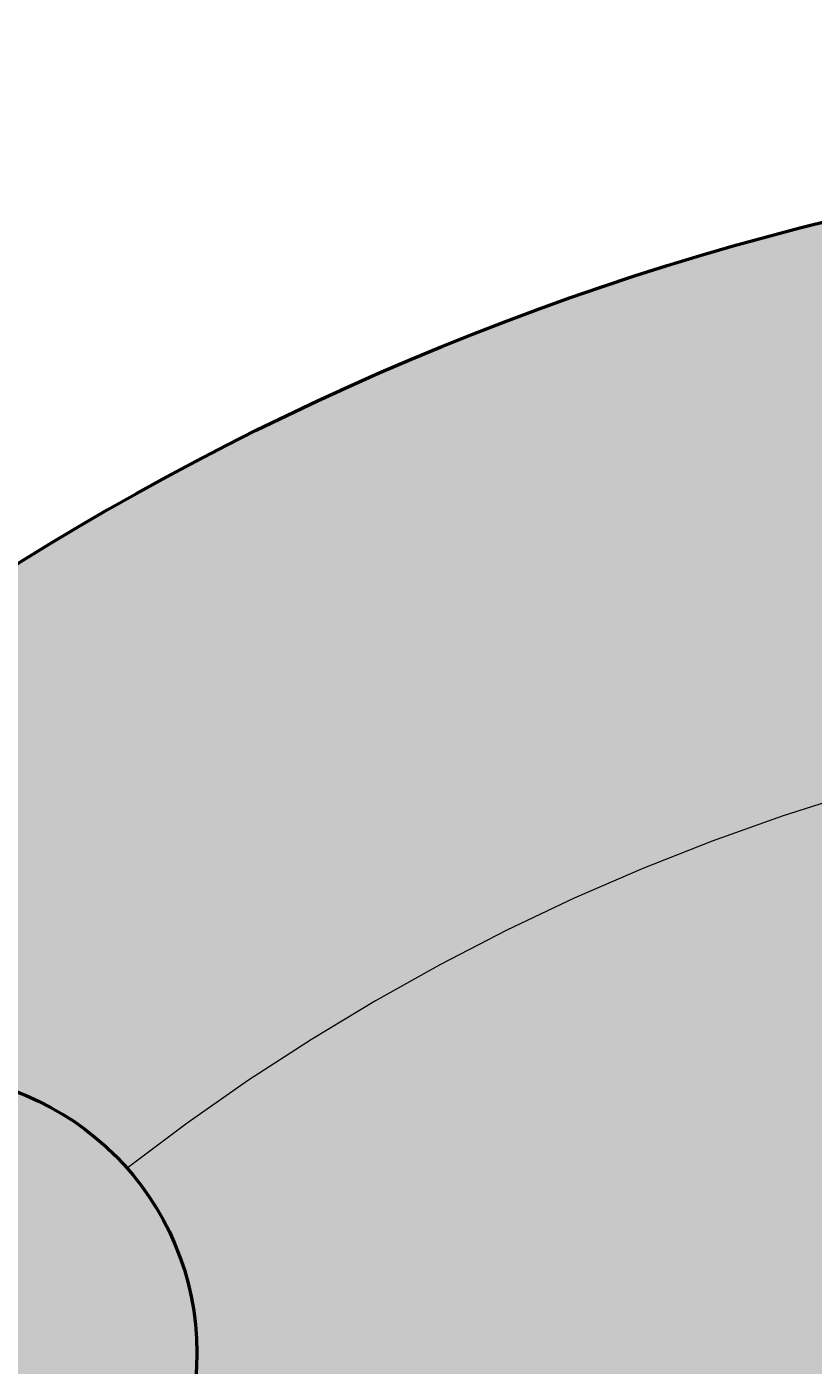
# Model space of a CAD drawing. Units: inches. Extents: x 139261 to 139415, y 52839 to 52963.
# Tile 17 of 20: x 139314 to 139328, y 52928 to 52952. Entities that reach past the tile are written whole.
import ezdxf

# ---------------------------------------------------------------- set-up
doc = ezdxf.new("R2010")
doc.units = ezdxf.units.IN
doc.header["$MEASUREMENT"] = 0
doc.linetypes.add('CENTER', pattern=[50.8, 31.75, -6.35, 6.35, -6.35])
for name, color, linetype, lineweight in [('M-CNTR', 4, 'CENTER', 18), ('M-DIMS', 2, 'Continuous', 25), ('M-HATC', 8, 'Continuous', 18), ('M-OUTL', 7, 'Continuous', 50)]:
    doc.layers.add(name, color=color, linetype=linetype, lineweight=lineweight)
doc.styles.get("Standard").update_dxf_attribs({"font": 'arial.ttf'})
doc.dimstyles.get("Standard").update_dxf_attribs({"dimtxt": 0.18, "dimasz": 0.18, "dimexe": 0.18, "dimexo": 0.0625, "dimgap": 0.09, "dimtad": 0, "dimtih": 1, "dimtoh": 1, "dimdec": 4, "dimzin": 0, "dimdsep": 46, "dimtxsty": 'Standard', "dimcen": 0.09, "dimadec": 0, "dimazin": 0, "dimtfac": 1, "dimtdec": 4, "dimtofl": 0, "dimtmove": 0, "dimatfit": 3, "dimfxl": 1, "dimtolj": 1, "dimtzin": 0, "dimarcsym": 0})

# ---------------------------------------------------------------- blocks, each defined once
blk = doc.blocks.new('*U1')
blk.add_circle((0, 0), 5)
blk = doc.blocks.new('*U2')
at = {"layer": 'M-OUTL', "color": 0, "linetype": 'ByBlock', "lineweight": -2, "transparency": 16777216, "rotation": 45.00000000000001}
blk.add_blockref('*U1', (139312.073, 52928.502), dxfattribs=at)
blk = doc.blocks.new('*D4')
at = {"layer": 'Defpoints', "color": 0, "transparency": 16777216}
for p in [(139373.053, 52923.26), (139307.661, 52877.175)]:
    blk.add_point(p, dxfattribs=at)
at = {"layer": 'M-DIMS', "color": 0, "lineweight": -2, "transparency": 16777216}
for p, q in [((139414.011, 52952.126), (139373.2, 52923.364)), ((139414.191, 52952.126), (139414.011, 52952.126)), ((139340.267, 52900.217), (139340.447, 52900.217)), ((139340.357, 52900.127), (139340.357, 52900.307))]:
    blk.add_line(p, q, dxfattribs=at)
blk.add_arc((139340.357, 52900.217), 40, 34.9168, 52.0771, dxfattribs=at)
at = {"layer": 'M-DIMS', "color": 0, "transparency": 16777216}
blk.add_solid([(139373.183, 52923.388), (139373.217, 52923.339), (139373.053, 52923.26)], dxfattribs=at)
at = {"layer": 'M-DIMS', "color": 0, "transparency": 16777216, "insert": (139414.822, 52952.126), "char_height": 0.18, "attachment_point": 5}
blk.add_mtext('\\A1;∅80.0000', dxfattribs=at)
blk = doc.blocks.new('*D9')
at = {"layer": 'Defpoints', "color": 0, "transparency": 16777216}
for p in [(139302.054, 52932.357), (139378.659, 52868.078)]:
    blk.add_point(p, dxfattribs=at)
at = {"layer": 'M-DIMS', "color": 0, "lineweight": -2, "transparency": 16777216}
for p, q in [((139278.893, 52951.64), (139279.073, 52951.64)), ((139279.073, 52951.64), (139301.916, 52932.472)), ((139340.267, 52900.217), (139340.447, 52900.217)), ((139340.357, 52900.127), (139340.357, 52900.307))]:
    blk.add_line(p, q, dxfattribs=at)
at = {"layer": 'M-DIMS', "color": 0, "transparency": 16777216}
blk.add_solid([(139301.936, 52932.495), (139301.897, 52932.449), (139302.054, 52932.357)], dxfattribs=at)
at = {"layer": 'M-DIMS', "color": 0, "transparency": 16777216, "insert": (139278.506, 52951.64), "char_height": 0.18, "attachment_point": 5}
blk.add_mtext('\\A1;∅100', dxfattribs=at)
blk = doc.blocks.new('*D10')
at = {"layer": 'Defpoints', "color": 0, "transparency": 16777216}
for p in [(139325.07, 52937.181), (139355.644, 52863.254)]:
    blk.add_point(p, dxfattribs=at)
at = {"layer": 'M-DIMS', "color": 0, "lineweight": -2, "transparency": 16777216}
for p, q in [((139340.267, 52900.217), (139340.447, 52900.217)), ((139340.357, 52900.127), (139340.357, 52900.307)), ((139364.816, 52841.075), (139355.712, 52863.087)), ((139364.996, 52841.075), (139364.816, 52841.075))]:
    blk.add_line(p, q, dxfattribs=at)
at = {"layer": 'M-DIMS', "color": 0, "transparency": 16777216}
blk.add_solid([(139355.74, 52863.099), (139355.685, 52863.076), (139355.644, 52863.254)], dxfattribs=at)
at = {"layer": 'M-DIMS', "color": 0, "transparency": 16777216, "insert": (139365.312, 52841.075), "char_height": 0.18, "attachment_point": 5}
blk.add_mtext('\\A1;∅80', dxfattribs=at)

msp = doc.modelspace()

# ---------------------------------------------------------------- hatches: boundary and pattern name
at = {"layer": 'M-HATC'}
h = msp.add_hatch(color=256, dxfattribs=at)
h.dxf.hatch_style = 1
h.paths.add_polyline_path([(139290.35689, 52900.21749, 1), (139390.35689, 52900.21749, 1)])
h.paths.add_polyline_path([(139335.36666, 52939.90499, -0.01563646), (139335.35689, 52940.21749, -1), (139345.35689, 52940.21749, -0.01563646), (139345.34711, 52939.90499, -0.13461315), (139364.89157, 52931.80941, -0.691035), (139373.64116, 52928.50176, -0.21521822), (139371.94881, 52924.75216, -0.13461315), (139380.04439, 52905.20771, -0.43265224), (139385.35689, 52900.21749, -0.43265224), (139380.04439, 52895.22726, -0.13461315), (139371.94881, 52875.68281, -0.21521822), (139373.64116, 52871.93321, -0.691035), (139364.89157, 52868.62556, -0.13461315), (139345.34711, 52860.52999, -0.01563646), (139345.35689, 52860.21749, -1), (139335.35689, 52860.21749, -0.01563646), (139335.36666, 52860.52999, -0.13461315), (139315.82221, 52868.62556, -0.691035), (139307.07262, 52871.93321, -0.21521822), (139308.76496, 52875.68281, -0.13461315), (139300.66939, 52895.22726, -0.43265224), (139295.35689, 52900.21749, -0.43265224), (139300.66939, 52905.20771, -0.13461315), (139308.76496, 52924.75216, -0.21521822), (139307.07262, 52928.50176, -0.691035), (139315.82221, 52931.80941, -0.13461315)], flags=16)
h.paths.add_polyline_path([(139365.35689, 52900.21749, -1), (139315.35689, 52900.21749, -1)], flags=0)
h.paths.add_polyline_path([(139323.71474, 52911.30978), (139356.99903, 52911.30978, -0.3027197), (139356.99903, 52889.12519), (139323.71474, 52889.12519, -0.3027197)], flags=0)
h.paths.add_polyline_path([(139364.89157, 52931.80941, 0.13461315), (139345.34711, 52939.90499, -0.93933644), (139335.36666, 52939.90499, 0.13461315), (139315.82221, 52931.80941, -0.18270763), (139317.07262, 52928.50176, -0.64579494), (139308.76496, 52924.75216, 0.13461315), (139300.66939, 52905.20771, -0.39601219), (139305.35689, 52900.21749, -0.39601219), (139300.66939, 52895.22726, 0.13461315), (139308.76496, 52875.68281, -0.64579494), (139317.07262, 52871.93321, -0.18270763), (139315.82221, 52868.62556, 0.13461315), (139335.36666, 52860.52999, -0.93933644), (139345.34711, 52860.52999, 0.13461315), (139364.89157, 52868.62556, -0.18270763), (139363.64116, 52871.93321, -0.64579494), (139371.94881, 52875.68281, 0.13461315), (139380.04439, 52895.22726, -0.39601219), (139375.35689, 52900.21749, -0.39601219), (139380.04439, 52905.20771, 0.13461315), (139371.94881, 52924.75216, -0.64579494), (139363.64116, 52928.50176, -0.18270763)], flags=0)
h = msp.add_hatch(color=256, dxfattribs=at)
h.dxf.hatch_style = 1
h.set_gradient(color1=(205, 105, 40), tint=1)
h.paths.add_polyline_path([(139335.35689, 52940.21749, 1), (139345.35689, 52940.21749, 1)])
h.paths.add_polyline_path([(139307.07262, 52928.50176, 1), (139317.07262, 52928.50176, 1)])
h.paths.add_polyline_path([(139295.35689, 52900.21749, 1), (139305.35689, 52900.21749, 1)])
h.paths.add_polyline_path([(139307.07262, 52871.93321, 1), (139317.07262, 52871.93321, 1)])
h.paths.add_polyline_path([(139345.35689, 52860.21749, 1), (139335.35689, 52860.21749, 1)])
h.paths.add_polyline_path([(139363.64116, 52871.93321, 1), (139373.64116, 52871.93321, 1)])
h.paths.add_polyline_path([(139375.35689, 52900.21749, 1), (139385.35689, 52900.21749, 1)])
h.paths.add_polyline_path([(139363.64116, 52928.50176, 1), (139373.64116, 52928.50176, 1)])
h = msp.add_hatch(color=256, dxfattribs=at)
h.dxf.hatch_style = 1
h.paths.add_polyline_path([(139345.34711, 52939.90499, -0.93933644), (139335.36666, 52939.90499, 0.13461315), (139315.82221, 52931.80941, -0.18270763), (139317.07262, 52928.50176, -0.64579494), (139308.76496, 52924.75216, 0.13461315), (139300.66939, 52905.20771, -0.39601219), (139305.35689, 52900.21749, -0.39601219), (139300.66939, 52895.22726, 0.13461315), (139308.76496, 52875.68281, -0.64579494), (139317.07262, 52871.93321, -0.18270763), (139315.82221, 52868.62556, 0.13461315), (139335.36666, 52860.52999, -0.93933644), (139345.34711, 52860.52999, 0.13461315), (139364.89157, 52868.62556, -0.18270763), (139363.64116, 52871.93321, -0.64579494), (139371.94881, 52875.68281, 0.13461315), (139380.04439, 52895.22726, -0.39601219), (139375.35689, 52900.21749, -0.39601219), (139380.04439, 52905.20771, 0.13461315), (139371.94881, 52924.75216, -0.64579494), (139363.64116, 52928.50176, -0.18270763), (139364.89157, 52931.80941, 0.13461315)])
h.paths.add_polyline_path([(139365.35689, 52900.21749, -1), (139315.35689, 52900.21749, -1)], flags=16)
h.paths.add_polyline_path([(139356.99903, 52911.30978, -0.3027197), (139356.99903, 52889.12519), (139323.71474, 52889.12519, -0.3027197), (139323.71474, 52911.30978)], flags=0)

# ---------------------------------------------------------------- linework, layer by layer
at = {"layer": 'M-CNTR'}
msp.add_arc((139340.35689, 52900.21749), 40, 97.166643, 127.833357, dxfattribs=at)
at = {"layer": 'M-OUTL'}
msp.add_circle((139340.35689, 52900.21749), 50, dxfattribs=at)

# ---------------------------------------------------------------- block references
msp.add_blockref('*U2', (0, 0), dxfattribs=at)

# ---------------------------------------------------------------- dimensions: what is measured, and where the dimension line sits
at = {"layer": 'M-DIMS'}
for p1, p2, override, picture, middle in [((139307.66087, 52877.17469), (139373.0529, 52923.26028), {"dimclrd": 0, "dimclre": 0, "dimclrt": 0}, '*D4', (139414.82217, 52952.12585)), ((139378.65939, 52868.07845), (139302.05438, 52932.35652), {"dimdec": 0, "dimlfac": 1, "dimrnd": 0, "dimzin": 0, "dimdsep": 46, "dimlunit": 2}, '*D9', (139278.50641, 52951.63995)), ((139325.07023, 52937.18123), (139355.64354, 52863.25374), {"dimdec": 0, "dimlfac": 1, "dimrnd": 0, "dimzin": 0, "dimdsep": 46, "dimlunit": 2}, '*D10', (139365.31206, 52841.0755))]:
    dim = msp.add_diameter_dim_2p(p1=p1, p2=p2, dimstyle='Standard', override=override, dxfattribs=at)
    dim.commit()
    dim.dimension.update_dxf_attribs({"geometry": picture, "text_midpoint": middle, "dimtype": 163})

doc.saveas('drawing.dxf')
